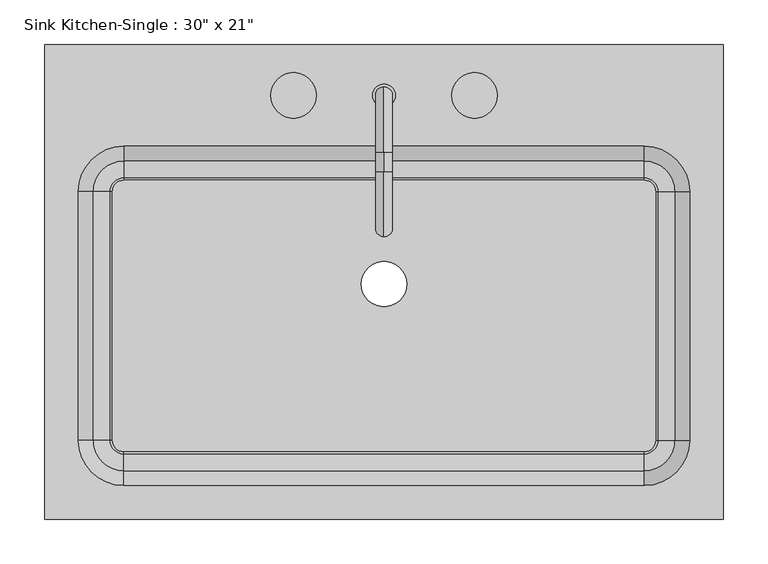
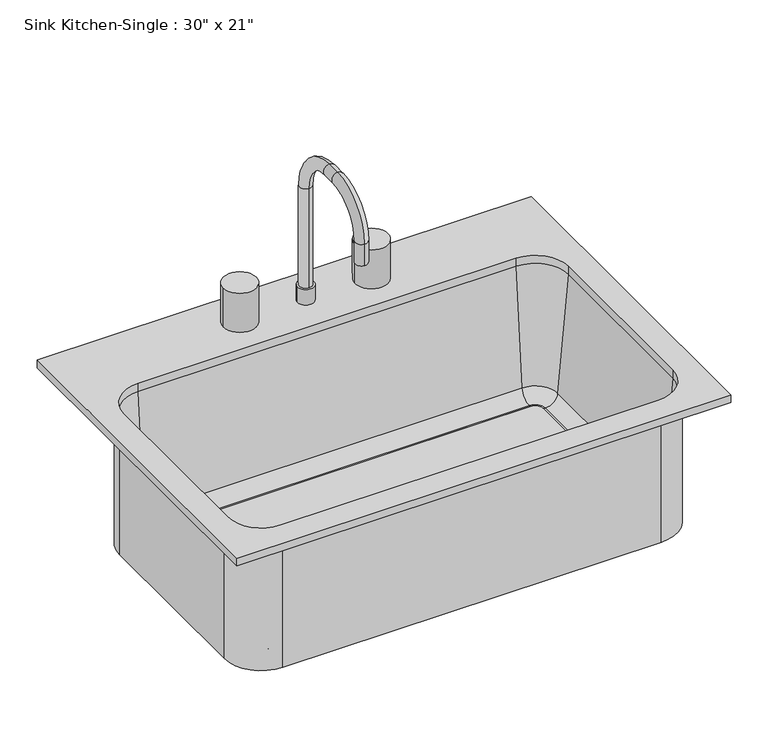
"""IFC4 building model written with IfcOpenShell, lengths in millimetres: flow terminal geometry."""

from ifc_helpers import new_model, si_unit, point, frame, frame_2d, origin, place, context, project, spatial, polyline, circle_curve, ellipse_curve, trimmed, segment, composite_curve, outline, extrude, source, transform, mapped, element, save
from ifc_brep_helpers import plane_surface, cylinder_surface, revolved_surface, advanced_brep


def flow_terminal_4d548711(model_context):
    return source(origin(), model_context, "Body", "SolidModel", [
        extrude(outline(composite_curve([segment(trimmed(circle_curve(frame_2d((307.7892406, 103.9454011)), 12.7), [point((307.7892406, 116.6454011))], [point((320.4892406, 103.9454011))], False, "CARTESIAN"), True, "CONTINUOUS"), segment(polyline([(320.4892406, 103.9454011), (320.4892406, -175.4545989)]), True, "CONTINUOUS"), segment(trimmed(circle_curve(frame_2d((307.7892406, -175.4545989)), 12.7), [point((320.4892406, -175.4545989))], [point((307.7892406, -188.1545989))], False, "CARTESIAN"), True, "CONTINUOUS"), segment(polyline([(307.7892406, -188.1545989), (-276.4107594, -188.1545989)]), True, "CONTINUOUS"), segment(trimmed(circle_curve(frame_2d((-276.4107594, -175.4545989)), 12.7), [point((-276.4107594, -188.1545989))], [point((-289.1107594, -175.4545989))], False, "CARTESIAN"), True, "CONTINUOUS"), segment(polyline([(-289.1107594, -175.4545989), (-289.1107594, 103.9454011)]), True, "CONTINUOUS"), segment(trimmed(circle_curve(frame_2d((-276.4107594, 103.9454011)), 12.7), [point((-289.1107594, 103.9454011))], [point((-276.4107594, 116.6454011))], False, "CARTESIAN"), True, "CONTINUOUS"), segment(polyline([(-276.4107594, 116.6454011), (307.7892406, 116.6454011)]), True, "CONTINUOUS")], self_intersect=False), holes=[composite_curve([segment(trimmed(circle_curve(frame_2d((15.6892406, 0.0)), 25.4), [point((-9.7107594, 0.0))], [point((41.0892406, 0.0))], True, "CARTESIAN"), True, "CONTINUOUS"), segment(trimmed(circle_curve(frame_2d((15.6892406, 0.0)), 25.4), [point((41.0892406, 0.0))], [point((-9.7107594, 0.0))], True, "CARTESIAN"), True, "CONTINUOUS")], self_intersect=False)]), frame((0.0, 0.0, 698.5), z_axis=(0.0, 0.0, 1.0), x_axis=(1.0, 0.0, 0.0)), (0.0, 0.0, 1.0), 9.525),
        extrude(outline(composite_curve([segment(trimmed(circle_curve(frame_2d((-85.9107594, 211.8954011)), 25.4), [point((-111.3107594, 211.8954011))], [point((-60.5107594, 211.8954011))], False, "CARTESIAN"), True, "CONTINUOUS"), segment(trimmed(circle_curve(frame_2d((-85.9107594, 211.8954011)), 25.4), [point((-60.5107594, 211.8954011))], [point((-111.3107594, 211.8954011))], False, "CARTESIAN"), True, "CONTINUOUS")], self_intersect=False)), frame((0.0, 0.0, 927.1), z_axis=(0.0, 0.0, 1.0), x_axis=(1.0, 0.0, 0.0)), (0.0, 0.0, 1.0), 63.5),
        extrude(outline(composite_curve([segment(trimmed(circle_curve(frame_2d((117.2892406, 211.8954011)), 25.4), [point((91.8892406, 211.8954011))], [point((142.6892406, 211.8954011))], False, "CARTESIAN"), True, "CONTINUOUS"), segment(trimmed(circle_curve(frame_2d((117.2892406, 211.8954011)), 25.4), [point((142.6892406, 211.8954011))], [point((91.8892406, 211.8954011))], False, "CARTESIAN"), True, "CONTINUOUS")], self_intersect=False)), frame((0.0, 0.0, 927.1), z_axis=(0.0, 0.0, 1.0), x_axis=(1.0, 0.0, 0.0)), (0.0, 0.0, 1.0), 63.5),
        advanced_brep(
        [(2.9892406, 211.8954011, 927.1), (28.3892406, 211.8954011, 927.1), (15.6892406, 221.4204011, 1114.425), (15.6892406, 202.3704011, 1114.425), (15.6892406, 202.3704011, 952.5), (15.6892406, 221.4204011, 952.5), (15.6892406, 148.3954011, 1187.45), (15.6892406, 148.3954011, 1168.4), (15.6892406, 126.1704011, 1187.45), (15.6892406, 126.1704011, 1168.4), (15.6892406, 53.1454011, 1114.425), (15.6892406, 72.1954011, 1114.425), (15.6892406, 53.1454011, 1079.5), (15.6892406, 72.1954011, 1079.5), (2.9892406, 211.8954011, 952.5), (28.3892406, 211.8954011, 952.5)],
        [
            (0, 1, circle_curve(frame((15.6892406, 211.8954011, 927.1), z_axis=(0.0, 0.0, -1.0), x_axis=(1.0, 0.0, 0.0)), 12.7)),
            (1, 0, circle_curve(frame((15.6892406, 211.8954011, 927.1), z_axis=(0.0, 0.0, -1.0), x_axis=(1.0, 0.0, 0.0)), 12.7)),
            (2, 3, circle_curve(frame((15.6892406, 211.8954011, 1114.425), z_axis=(0.0, 0.0, -1.0), x_axis=(0.0, -1.0, 0.0)), 9.525)),
            (3, 4),
            (4, 5, circle_curve(frame((15.6892406, 211.8954011, 952.5), z_axis=(0.0, 0.0, 1.0), x_axis=(0.0, -1.0, 0.0)), 9.525)),
            (5, 2),
            (3, 2, circle_curve(frame((15.6892406, 211.8954011, 1114.425), z_axis=(0.0, 0.0, -1.0), x_axis=(0.0, -1.0, 0.0)), 9.525)),
            (5, 4, circle_curve(frame((15.6892406, 211.8954011, 952.5), z_axis=(0.0, 0.0, 1.0), x_axis=(0.0, -1.0, 0.0)), 9.525)),
            (2, 6, circle_curve(frame((15.6892406, 148.3954011, 1114.425), z_axis=(1.0, 0.0, 0.0), x_axis=(0.0, 1.0, 0.0)), 73.025)),
            (6, 7, circle_curve(frame((15.6892406, 148.3954011, 1177.925), z_axis=(0.0, 1.0, 0.0), x_axis=(0.0, 0.0, -1.0)), 9.525)),
            (7, 3, circle_curve(frame((15.6892406, 148.3954011, 1114.425), z_axis=(-1.0, 0.0, 0.0), x_axis=(0.0, 1.0, 0.0)), 53.975)),
            (7, 6, circle_curve(frame((15.6892406, 148.3954011, 1177.925), z_axis=(0.0, 1.0, 0.0), x_axis=(0.0, 0.0, -1.0)), 9.525)),
            (6, 8),
            (8, 9, circle_curve(frame((15.6892406, 126.1704011, 1177.925), z_axis=(0.0, 1.0, 0.0), x_axis=(0.0, 0.0, -1.0)), 9.525)),
            (9, 7),
            (9, 8, circle_curve(frame((15.6892406, 126.1704011, 1177.925), z_axis=(0.0, 1.0, 0.0), x_axis=(0.0, 0.0, -1.0)), 9.525)),
            (8, 10, circle_curve(frame((15.6892406, 126.1704011, 1114.425), z_axis=(1.0, 0.0, 0.0), x_axis=(0.0, 0.0, 1.0)), 73.025)),
            (10, 11, circle_curve(frame((15.6892406, 62.6704011, 1114.425), z_axis=(0.0, 0.0, 1.0), x_axis=(0.0, 1.0, 0.0)), 9.525)),
            (11, 9, circle_curve(frame((15.6892406, 126.1704011, 1114.425), z_axis=(-1.0, 0.0, 0.0), x_axis=(0.0, 0.0, 1.0)), 53.975)),
            (11, 10, circle_curve(frame((15.6892406, 62.6704011, 1114.425), z_axis=(0.0, 0.0, 1.0), x_axis=(0.0, 1.0, 0.0)), 9.525)),
            (12, 13, circle_curve(frame((15.6892406, 62.6704011, 1079.5), z_axis=(0.0, 0.0, -1.0), x_axis=(0.0, 1.0, 0.0)), 9.525)),
            (13, 12, circle_curve(frame((15.6892406, 62.6704011, 1079.5), z_axis=(0.0, 0.0, -1.0), x_axis=(0.0, 1.0, 0.0)), 9.525)),
            (10, 12),
            (13, 11),
            (14, 15, circle_curve(frame((15.6892406, 211.8954011, 952.5), z_axis=(0.0, 0.0, 1.0), x_axis=(1.0, 0.0, 0.0)), 12.7)),
            (15, 14, circle_curve(frame((15.6892406, 211.8954011, 952.5), z_axis=(0.0, 0.0, 1.0), x_axis=(1.0, 0.0, 0.0)), 12.7)),
            (14, 0),
            (1, 15),
        ],
        [
            plane_surface(frame((15.6892406, 202.3704011, 927.1), z_axis=(0.0, 0.0, -1.0), x_axis=(1.0, 0.0, 0.0))),
            cylinder_surface(frame((15.6892406, 211.8954011, 927.1), z_axis=(0.0, 0.0, -1.0), x_axis=(0.0, -1.0, 0.0)), 9.525),
            revolved_surface(trimmed(ellipse_curve(frame((15.6892406, 211.8954011, 1114.425), z_axis=(0.0, 0.0, -1.0), x_axis=(0.0, -1.0, 0.0)), 9.525, 9.525), [point((15.6892406, 221.4204011, 1114.425))], [point((15.6892406, 202.3704011, 1114.425))], True, "CARTESIAN"), (15.6892406, 148.3954011, 1114.425), (1.0, 0.0, 0.0)),
            revolved_surface(trimmed(ellipse_curve(frame((15.6892406, 211.8954011, 1114.425), z_axis=(0.0, 0.0, -1.0), x_axis=(0.0, -1.0, 0.0)), 9.525, 9.525), [point((15.6892406, 202.3704011, 1114.425))], [point((15.6892406, 221.4204011, 1114.425))], True, "CARTESIAN"), (15.6892406, 148.3954011, 1114.425), (1.0, 0.0, 0.0)),
            cylinder_surface(frame((15.6892406, 148.3954011, 1177.925), z_axis=(0.0, 1.0, 0.0), x_axis=(0.0, 0.0, -1.0)), 9.525),
            revolved_surface(trimmed(ellipse_curve(frame((15.6892406, 126.1704011, 1177.925), z_axis=(0.0, 1.0, 0.0), x_axis=(0.0, 0.0, -1.0)), 9.525, 9.525), [point((15.6892406, 126.1704011, 1187.45))], [point((15.6892406, 126.1704011, 1168.4))], True, "CARTESIAN"), (15.6892406, 126.1704011, 1114.425), (1.0, 0.0, 0.0)),
            revolved_surface(trimmed(ellipse_curve(frame((15.6892406, 126.1704011, 1177.925), z_axis=(0.0, 1.0, 0.0), x_axis=(0.0, 0.0, -1.0)), 9.525, 9.525), [point((15.6892406, 126.1704011, 1168.4))], [point((15.6892406, 126.1704011, 1187.45))], True, "CARTESIAN"), (15.6892406, 126.1704011, 1114.425), (1.0, 0.0, 0.0)),
            plane_surface(frame((15.6892406, 53.1454011, 1079.5), z_axis=(0.0, 0.0, -1.0), x_axis=(-1.0, 0.0, 0.0))),
            cylinder_surface(frame((15.6892406, 62.6704011, 1114.425), z_axis=(0.0, 0.0, 1.0), x_axis=(0.0, 1.0, 0.0)), 9.525),
            plane_surface(frame((28.3892406, 211.8954011, 952.5), z_axis=(0.0, 0.0, 1.0), x_axis=(0.0, 1.0, 0.0))),
            cylinder_surface(frame((15.6892406, 211.8954011, 927.1), z_axis=(0.0, 0.0, 1.0), x_axis=(1.0, 0.0, 0.0)), 12.7),
        ],
        [
            (0, [[1, 2]]),
            (1, [[3, 4, 5, 6]]),
            (1, [[7, -6, 8, -4]]),
            (2, [[-3, 9, 10, 11]]),
            (3, [[-7, -11, 12, -9]]),
            (4, [[-10, 13, 14, 15]]),
            (4, [[-12, -15, 16, -13]]),
            (5, [[-14, 17, 18, 19]]),
            (6, [[-16, -19, 20, -17]]),
            (7, [[21, 22]]),
            (8, [[-18, 23, -22, 24]]),
            (8, [[-20, -24, -21, -23]]),
            (9, [[25, 26], [-5, -8]]),
            (10, [[-25, 27, -2, 28]]),
            (10, [[-26, -28, -1, -27]]),
        ],
    ),
        advanced_brep(
        [(396.6892406, 269.0454011, 927.1), (-365.3107594, 269.0454011, 927.1), (-365.3107594, -264.3545989, 927.1), (396.6892406, -264.3545989, 927.1), (307.7892406, 154.7454011, 927.1), (358.5892406, 103.9454011, 927.1), (358.5892406, -175.4545989, 927.1), (307.7892406, -226.2545989, 927.1), (-276.4107594, -226.2545989, 927.1), (-327.2107594, -175.4545989, 927.1), (-327.2107594, 103.9454011, 927.1), (-276.4107594, 154.7454011, 927.1), (396.6892406, 269.0454011, 914.4), (396.6892406, -264.3545989, 914.4), (-365.3107594, -264.3545989, 914.4), (-365.3107594, 269.0454011, 914.4), (364.9392406, 103.9454011, 914.4), (307.7892406, 161.0954011, 914.4), (-276.4107594, 161.0954011, 914.4), (-333.5607594, 103.9454011, 914.4), (-333.5607594, -175.4545989, 914.4), (-276.4107594, -232.6045989, 914.4), (307.7892406, -232.6045989, 914.4), (364.9392406, -175.4545989, 914.4), (307.7892406, 154.7454011, 914.4), (358.5892406, 103.9454011, 914.4), (358.5892406, -175.4545989, 914.4), (307.7892406, -226.2545989, 914.4), (-276.4107594, -226.2545989, 914.4), (-327.2107594, -175.4545989, 914.4), (-327.2107594, 103.9454011, 914.4), (-276.4107594, 154.7454011, 914.4), (364.9392406, 103.9454011, 698.5), (307.7892406, 161.0954011, 698.5), (320.4892406, 103.9454011, 698.5), (307.7892406, 116.6454011, 698.5), (320.4892406, 103.9454011, 708.025), (307.7892406, 116.6454011, 708.025), (323.0776588, 103.9454011, 708.025), (307.7892406, 119.2338193, 708.025), (342.0551678, 103.9454011, 725.4146831), (307.7892406, 138.2113283, 725.4146831), (364.9392406, -175.4545989, 698.5), (320.4892406, -175.4545989, 698.5), (320.4892406, -175.4545989, 708.025), (323.0776588, -175.4545989, 708.025), (342.0551678, -175.4545989, 725.4146831), (307.7892406, -232.6045989, 698.5), (307.7892406, -188.1545989, 698.5), (307.7892406, -188.1545989, 708.025), (307.7892406, -190.7430171, 708.025), (307.7892406, -209.7205261, 725.4146831), (-276.4107594, -232.6045989, 698.5), (-276.4107594, -188.1545989, 698.5), (-276.4107594, -188.1545989, 708.025), (-276.4107594, -190.7430171, 708.025), (-276.4107594, -209.7205261, 725.4146831), (-333.5607594, -175.4545989, 698.5), (-289.1107594, -175.4545989, 698.5), (-289.1107594, -175.4545989, 708.025), (-291.6991776, -175.4545989, 708.025), (-310.6766866, -175.4545989, 725.4146831), (-333.5607594, 103.9454011, 698.5), (-289.1107594, 103.9454011, 698.5), (-289.1107594, 103.9454011, 708.025), (-291.6991776, 103.9454011, 708.025), (-310.6766866, 103.9454011, 725.4146831), (-276.4107594, 161.0954011, 698.5), (-276.4107594, 116.6454011, 698.5), (-276.4107594, 116.6454011, 708.025), (-276.4107594, 119.2338193, 708.025), (-276.4107594, 138.2113283, 725.4146831)],
        [
            (0, 1),
            (1, 2),
            (2, 3),
            (3, 0),
            (4, 5, circle_curve(frame((307.7892406, 103.9454011, 927.1), z_axis=(0.0, 0.0, -1.0), x_axis=(1.0, 0.0, 0.0)), 50.8)),
            (5, 6),
            (6, 7, circle_curve(frame((307.7892406, -175.4545989, 927.1), z_axis=(0.0, 0.0, -1.0), x_axis=(1.0, 0.0, 0.0)), 50.8)),
            (7, 8),
            (8, 9, circle_curve(frame((-276.4107594, -175.4545989, 927.1), z_axis=(0.0, 0.0, -1.0), x_axis=(1.0, 0.0, 0.0)), 50.8)),
            (9, 10),
            (10, 11, circle_curve(frame((-276.4107594, 103.9454011, 927.1), z_axis=(0.0, 0.0, -1.0), x_axis=(1.0, 0.0, 0.0)), 50.8)),
            (11, 4),
            (12, 13),
            (13, 14),
            (14, 15),
            (15, 12),
            (16, 17, circle_curve(frame((307.7892406, 103.9454011, 914.4), z_axis=(0.0, 0.0, 1.0), x_axis=(0.0, 1.0, 0.0)), 57.15)),
            (17, 18),
            (18, 19, circle_curve(frame((-276.4107594, 103.9454011, 914.4), z_axis=(0.0, 0.0, 1.0), x_axis=(-1.0, 0.0, 0.0)), 57.15)),
            (19, 20),
            (20, 21, circle_curve(frame((-276.4107594, -175.4545989, 914.4), z_axis=(0.0, 0.0, 1.0), x_axis=(0.0, -1.0, 0.0)), 57.15)),
            (21, 22),
            (22, 23, circle_curve(frame((307.7892406, -175.4545989, 914.4), z_axis=(0.0, 0.0, 1.0), x_axis=(1.0, 0.0, 0.0)), 57.15)),
            (23, 16),
            (0, 12),
            (15, 1),
            (14, 2),
            (13, 3),
            (4, 24),
            (24, 25, circle_curve(frame((307.7892406, 103.9454011, 914.4), z_axis=(0.0, 0.0, -1.0), x_axis=(1.0, 0.0, 0.0)), 50.8)),
            (25, 5),
            (25, 26),
            (26, 6),
            (26, 27, circle_curve(frame((307.7892406, -175.4545989, 914.4), z_axis=(0.0, 0.0, -1.0), x_axis=(1.0, 0.0, 0.0)), 50.8)),
            (27, 7),
            (27, 28),
            (28, 8),
            (28, 29, circle_curve(frame((-276.4107594, -175.4545989, 914.4), z_axis=(0.0, 0.0, -1.0), x_axis=(1.0, 0.0, 0.0)), 50.8)),
            (29, 9),
            (29, 30),
            (30, 10),
            (30, 31, circle_curve(frame((-276.4107594, 103.9454011, 914.4), z_axis=(0.0, 0.0, -1.0), x_axis=(1.0, 0.0, 0.0)), 50.8)),
            (31, 11),
            (31, 24),
            (32, 33, circle_curve(frame((307.7892406, 103.9454011, 698.5), z_axis=(0.0, 0.0, 1.0), x_axis=(0.0, 1.0, 0.0)), 57.15)),
            (33, 17),
            (16, 32),
            (32, 34),
            (34, 35, circle_curve(frame((307.7892406, 103.9454011, 698.5), z_axis=(0.0, 0.0, 1.0), x_axis=(0.0, 1.0, 0.0)), 12.7)),
            (35, 33),
            (34, 36),
            (36, 37, circle_curve(frame((307.7892406, 103.9454011, 708.025), z_axis=(0.0, 0.0, 1.0), x_axis=(0.0, 1.0, 0.0)), 12.7)),
            (37, 35),
            (36, 38),
            (38, 39, circle_curve(frame((307.7892406, 103.9454011, 708.025), z_axis=(0.0, 0.0, 1.0), x_axis=(0.0, 1.0, 0.0)), 15.2884182)),
            (39, 37),
            (38, 40, circle_curve(frame((323.0776588, 103.9454011, 727.075), z_axis=(0.0, -1.0, 0.0), x_axis=(1.0, 0.0, 0.0)), 19.05)),
            (40, 41, circle_curve(frame((307.7892406, 103.9454011, 725.4146831), z_axis=(0.0, 0.0, 1.0), x_axis=(0.0, 1.0, 0.0)), 34.2659272)),
            (41, 39, circle_curve(frame((307.7892406, 119.2338193, 727.075), z_axis=(-1.0, 0.0, 0.0), x_axis=(0.0, 1.0, 0.0)), 19.05)),
            (40, 25),
            (24, 41),
            (23, 42),
            (42, 32),
            (42, 43),
            (43, 34),
            (43, 44),
            (44, 36),
            (44, 45),
            (45, 38),
            (45, 46, circle_curve(frame((323.0776588, -175.4545989, 727.075), z_axis=(0.0, -1.0, 0.0), x_axis=(1.0, 0.0, 0.0)), 19.05)),
            (46, 40),
            (46, 26),
            (22, 47),
            (47, 42, circle_curve(frame((307.7892406, -175.4545989, 698.5), z_axis=(0.0, 0.0, 1.0), x_axis=(1.0, 0.0, 0.0)), 57.15)),
            (47, 48),
            (48, 43, circle_curve(frame((307.7892406, -175.4545989, 698.5), z_axis=(0.0, 0.0, 1.0), x_axis=(1.0, 0.0, 0.0)), 12.7)),
            (48, 49),
            (49, 44, circle_curve(frame((307.7892406, -175.4545989, 708.025), z_axis=(0.0, 0.0, 1.0), x_axis=(1.0, 0.0, 0.0)), 12.7)),
            (49, 50),
            (50, 45, circle_curve(frame((307.7892406, -175.4545989, 708.025), z_axis=(0.0, 0.0, 1.0), x_axis=(1.0, 0.0, 0.0)), 15.2884182)),
            (50, 51, circle_curve(frame((307.7892406, -190.7430171, 727.075), z_axis=(-1.0, 0.0, 0.0), x_axis=(0.0, -1.0, 0.0)), 19.05)),
            (51, 46, circle_curve(frame((307.7892406, -175.4545989, 725.4146831), z_axis=(0.0, 0.0, 1.0), x_axis=(1.0, 0.0, 0.0)), 34.2659272)),
            (51, 27),
            (21, 52),
            (52, 47),
            (52, 53),
            (53, 48),
            (53, 54),
            (54, 49),
            (54, 55),
            (55, 50),
            (55, 56, circle_curve(frame((-276.4107594, -190.7430171, 727.075), z_axis=(-1.0, 0.0, 0.0), x_axis=(0.0, -1.0, 0.0)), 19.05)),
            (56, 51),
            (56, 28),
            (20, 57),
            (57, 52, circle_curve(frame((-276.4107594, -175.4545989, 698.5), z_axis=(0.0, 0.0, 1.0), x_axis=(0.0, -1.0, 0.0)), 57.15)),
            (57, 58),
            (58, 53, circle_curve(frame((-276.4107594, -175.4545989, 698.5), z_axis=(0.0, 0.0, 1.0), x_axis=(0.0, -1.0, 0.0)), 12.7)),
            (58, 59),
            (59, 54, circle_curve(frame((-276.4107594, -175.4545989, 708.025), z_axis=(0.0, 0.0, 1.0), x_axis=(0.0, -1.0, 0.0)), 12.7)),
            (59, 60),
            (60, 55, circle_curve(frame((-276.4107594, -175.4545989, 708.025), z_axis=(0.0, 0.0, 1.0), x_axis=(0.0, -1.0, 0.0)), 15.2884182)),
            (60, 61, circle_curve(frame((-291.6991776, -175.4545989, 727.075), z_axis=(0.0, 1.0, 0.0), x_axis=(-1.0, 0.0, 0.0)), 19.05)),
            (61, 56, circle_curve(frame((-276.4107594, -175.4545989, 725.4146831), z_axis=(0.0, 0.0, 1.0), x_axis=(0.0, -1.0, 0.0)), 34.2659272)),
            (61, 29),
            (19, 62),
            (62, 57),
            (62, 63),
            (63, 58),
            (63, 64),
            (64, 59),
            (64, 65),
            (65, 60),
            (65, 66, circle_curve(frame((-291.6991776, 103.9454011, 727.075), z_axis=(0.0, 1.0, 0.0), x_axis=(-1.0, 0.0, 0.0)), 19.05)),
            (66, 61),
            (66, 30),
            (18, 67),
            (67, 62, circle_curve(frame((-276.4107594, 103.9454011, 698.5), z_axis=(0.0, 0.0, 1.0), x_axis=(-1.0, 0.0, 0.0)), 57.15)),
            (67, 68),
            (68, 63, circle_curve(frame((-276.4107594, 103.9454011, 698.5), z_axis=(0.0, 0.0, 1.0), x_axis=(-1.0, 0.0, 0.0)), 12.7)),
            (68, 69),
            (69, 64, circle_curve(frame((-276.4107594, 103.9454011, 708.025), z_axis=(0.0, 0.0, 1.0), x_axis=(-1.0, 0.0, 0.0)), 12.7)),
            (69, 70),
            (70, 65, circle_curve(frame((-276.4107594, 103.9454011, 708.025), z_axis=(0.0, 0.0, 1.0), x_axis=(-1.0, 0.0, 0.0)), 15.2884182)),
            (70, 71, circle_curve(frame((-276.4107594, 119.2338193, 727.075), z_axis=(1.0, 0.0, 0.0), x_axis=(0.0, 1.0, 0.0)), 19.05)),
            (71, 66, circle_curve(frame((-276.4107594, 103.9454011, 725.4146831), z_axis=(0.0, 0.0, 1.0), x_axis=(-1.0, 0.0, 0.0)), 34.2659272)),
            (71, 31),
            (33, 67),
            (35, 68),
            (37, 69),
            (39, 70),
            (41, 71),
        ],
        [
            plane_surface(frame((-365.3107594, 269.0454011, 927.1), z_axis=(0.0, 0.0, 1.0), x_axis=(-1.0, 0.0, 0.0))),
            plane_surface(frame((-365.3107594, 269.0454011, 914.4), z_axis=(0.0, 0.0, -1.0), x_axis=(1.0, 0.0, 0.0))),
            plane_surface(frame((396.6892406, 269.0454011, 927.1), z_axis=(0.0, 1.0, 0.0), x_axis=(0.0, 0.0, -1.0))),
            plane_surface(frame((-365.3107594, 269.0454011, 927.1), z_axis=(-1.0, 0.0, 0.0), x_axis=(0.0, 0.0, -1.0))),
            plane_surface(frame((-365.3107594, -264.3545989, 927.1), z_axis=(0.0, -1.0, 0.0), x_axis=(0.0, 0.0, -1.0))),
            plane_surface(frame((396.6892406, -264.3545989, 927.1), z_axis=(1.0, 0.0, 0.0), x_axis=(0.0, 0.0, -1.0))),
            revolved_surface(polyline([(358.58924060000004, 103.9454011, 914.4), (358.58924060000004, 103.9454011, 927.1)]), (307.7892406, 103.9454011, 0.0), (0.0, 0.0, -1.0)),
            plane_surface(frame((358.5892406, 103.9454011, 927.1), z_axis=(-1.0, 0.0, 0.0), x_axis=(0.0, 0.0, -1.0))),
            revolved_surface(polyline([(358.58924060000004, -175.4545989, 914.4), (358.58924060000004, -175.4545989, 927.1)]), (307.7892406, -175.4545989, 0.0), (0.0, 0.0, -1.0)),
            plane_surface(frame((307.7892406, -226.2545989, 927.1), z_axis=(0.0, 1.0, 0.0), x_axis=(0.0, 0.0, -1.0))),
            revolved_surface(polyline([(-225.6107594, -175.4545989, 914.4), (-225.6107594, -175.4545989, 927.1)]), (-276.4107594, -175.4545989, 0.0), (0.0, 0.0, -1.0)),
            plane_surface(frame((-327.2107594, -175.4545989, 927.1), z_axis=(1.0, 0.0, 0.0), x_axis=(0.0, 0.0, -1.0))),
            revolved_surface(polyline([(-225.6107594, 103.9454011, 914.4), (-225.6107594, 103.9454011, 927.1)]), (-276.4107594, 103.9454011, 0.0), (0.0, 0.0, -1.0)),
            plane_surface(frame((-276.4107594, 154.7454011, 927.1), z_axis=(0.0, -1.0, 0.0), x_axis=(0.0, 0.0, -1.0))),
            cylinder_surface(frame((307.7892406, 103.9454011, 0.0), z_axis=(0.0, 0.0, -1.0), x_axis=(0.0, 1.0, 0.0)), 57.15),
            plane_surface(frame((307.7892406, 103.9454011, 698.5), z_axis=(0.0, 0.0, -1.0), x_axis=(0.0, 1.0, 0.0))),
            revolved_surface(polyline([(307.7892406, 116.6454011, 698.5), (307.7892406, 116.6454011, 708.025)]), (307.7892406, 103.9454011, 0.0), (0.0, 0.0, -1.0)),
            plane_surface(frame((307.7892406, 103.9454011, 708.025), z_axis=(0.0, 0.0, 1.0), x_axis=(0.0, 1.0, 0.0))),
            revolved_surface(trimmed(ellipse_curve(frame((307.7892406, 119.2338193, 727.075), z_axis=(1.0, 0.0, 0.0), x_axis=(0.0, 1.0, 0.0)), 19.05, 19.05), [point((307.7892406, 119.2338193, 708.025))], [point((307.7892406, 138.2113283, 725.4146831))], True, "CARTESIAN"), (307.7892406, 103.9454011, 0.0), (0.0, 0.0, -1.0)),
            revolved_surface(polyline([(307.7892406, 138.2113283, 725.4146831), (307.7892406, 154.7454011, 914.4)]), (307.7892406, 103.9454011, 0.0), (0.0, 0.0, -1.0)),
            plane_surface(frame((364.9392406, 103.9454011, 914.4), z_axis=(1.0, 0.0, 0.0), x_axis=(0.0, -1.0, 0.0))),
            plane_surface(frame((364.9392406, 103.9454011, 698.5), z_axis=(0.0, 0.0, -1.0), x_axis=(0.0, -1.0, 0.0))),
            plane_surface(frame((320.4892406, 103.9454011, 698.5), z_axis=(-1.0, 0.0, 0.0), x_axis=(0.0, -1.0, 0.0))),
            plane_surface(frame((320.4892406, 103.9454011, 708.025), z_axis=(0.0, 0.0, 1.0), x_axis=(0.0, -1.0, 0.0))),
            revolved_surface(polyline([(342.1276588, -175.45459889999998, 727.075), (342.1276588, 103.9454011, 727.075)]), (323.0776588, 103.9454011, 727.075), (0.0, -1.0, 0.0)),
            plane_surface(frame((342.0551678, 103.9454011, 725.4146831), z_axis=(-0.9961946980917442, 0.0, 0.08715574274767306), x_axis=(0.0, -1.0, 0.0))),
            cylinder_surface(frame((307.7892406, -175.4545989, 0.0), z_axis=(0.0, 0.0, -1.0), x_axis=(1.0, 0.0, 0.0)), 57.15),
            plane_surface(frame((307.7892406, -175.4545989, 698.5), z_axis=(0.0, 0.0, -1.0), x_axis=(1.0, 0.0, 0.0))),
            revolved_surface(polyline([(320.4892406, -175.4545989, 698.5), (320.4892406, -175.4545989, 708.025)]), (307.7892406, -175.4545989, 0.0), (0.0, 0.0, -1.0)),
            plane_surface(frame((307.7892406, -175.4545989, 708.025), z_axis=(0.0, 0.0, 1.0), x_axis=(1.0, 0.0, 0.0))),
            revolved_surface(trimmed(ellipse_curve(frame((323.0776588, -175.4545989, 727.075), z_axis=(0.0, -1.0, 0.0), x_axis=(1.0, 0.0, 0.0)), 19.05, 19.05), [point((323.0776588, -175.4545989, 708.025))], [point((342.0551678, -175.4545989, 725.4146831))], True, "CARTESIAN"), (307.7892406, -175.4545989, 0.0), (0.0, 0.0, -1.0)),
            revolved_surface(polyline([(342.0551678, -175.4545989, 725.4146831), (358.5892406, -175.4545989, 914.4)]), (307.7892406, -175.4545989, 0.0), (0.0, 0.0, -1.0)),
            plane_surface(frame((307.7892406, -232.6045989, 914.4), z_axis=(0.0, -1.0, 0.0), x_axis=(-1.0, 0.0, 0.0))),
            plane_surface(frame((307.7892406, -232.6045989, 698.5), z_axis=(0.0, 0.0, -1.0), x_axis=(-1.0, 0.0, 0.0))),
            plane_surface(frame((307.7892406, -188.1545989, 698.5), z_axis=(0.0, 1.0, 0.0), x_axis=(-1.0, 0.0, 0.0))),
            plane_surface(frame((307.7892406, -188.1545989, 708.025), z_axis=(0.0, 0.0, 1.0), x_axis=(-1.0, 0.0, 0.0))),
            revolved_surface(polyline([(-276.4107594, -209.79301710000001, 727.075), (307.7892406, -209.79301710000001, 727.075)]), (307.7892406, -190.7430171, 727.075), (-1.0, 0.0, 0.0)),
            plane_surface(frame((307.7892406, -209.7205261, 725.4146831), z_axis=(0.0, 0.9961946980917442, 0.08715574274767306), x_axis=(-1.0, 0.0, 0.0))),
            cylinder_surface(frame((-276.4107594, -175.4545989, 0.0), z_axis=(0.0, 0.0, -1.0), x_axis=(0.0, -1.0, 0.0)), 57.15),
            plane_surface(frame((-276.4107594, -175.4545989, 698.5), z_axis=(0.0, 0.0, -1.0), x_axis=(0.0, -1.0, 0.0))),
            revolved_surface(polyline([(-276.4107594, -188.1545989, 698.5), (-276.4107594, -188.1545989, 708.025)]), (-276.4107594, -175.4545989, 0.0), (0.0, 0.0, -1.0)),
            plane_surface(frame((-276.4107594, -175.4545989, 708.025), z_axis=(0.0, 0.0, 1.0), x_axis=(0.0, -1.0, 0.0))),
            revolved_surface(trimmed(ellipse_curve(frame((-276.4107594, -190.7430171, 727.075), z_axis=(-1.0, 0.0, 0.0), x_axis=(0.0, -1.0, 0.0)), 19.05, 19.05), [point((-276.4107594, -190.7430171, 708.025))], [point((-276.4107594, -209.7205261, 725.4146831))], True, "CARTESIAN"), (-276.4107594, -175.4545989, 0.0), (0.0, 0.0, -1.0)),
            revolved_surface(polyline([(-276.4107594, -209.7205261, 725.4146831), (-276.4107594, -226.2545989, 914.4)]), (-276.4107594, -175.4545989, 0.0), (0.0, 0.0, -1.0)),
            plane_surface(frame((-333.5607594, -175.4545989, 914.4), z_axis=(-1.0, 0.0, 0.0), x_axis=(0.0, 1.0, 0.0))),
            plane_surface(frame((-333.5607594, -175.4545989, 698.5), z_axis=(0.0, 0.0, -1.0), x_axis=(0.0, 1.0, 0.0))),
            plane_surface(frame((-289.1107594, -175.4545989, 698.5), z_axis=(1.0, 0.0, 0.0), x_axis=(0.0, 1.0, 0.0))),
            plane_surface(frame((-289.1107594, -175.4545989, 708.025), z_axis=(0.0, 0.0, 1.0), x_axis=(0.0, 1.0, 0.0))),
            revolved_surface(polyline([(-310.7491776, 103.94540109999997, 727.075), (-310.7491776, -175.4545989, 727.075)]), (-291.6991776, -175.4545989, 727.075), (0.0, 1.0, 0.0)),
            plane_surface(frame((-310.6766866, -175.4545989, 725.4146831), z_axis=(0.9961946980917442, 0.0, 0.08715574274767306), x_axis=(0.0, 1.0, 0.0))),
            cylinder_surface(frame((-276.4107594, 103.9454011, 0.0), z_axis=(0.0, 0.0, -1.0), x_axis=(-1.0, 0.0, 0.0)), 57.15),
            plane_surface(frame((-276.4107594, 103.9454011, 698.5), z_axis=(0.0, 0.0, -1.0), x_axis=(-1.0, 0.0, 0.0))),
            revolved_surface(polyline([(-289.1107594, 103.9454011, 698.5), (-289.1107594, 103.9454011, 708.025)]), (-276.4107594, 103.9454011, 0.0), (0.0, 0.0, -1.0)),
            plane_surface(frame((-276.4107594, 103.9454011, 708.025), z_axis=(0.0, 0.0, 1.0), x_axis=(-1.0, 0.0, 0.0))),
            revolved_surface(trimmed(ellipse_curve(frame((-291.6991776, 103.9454011, 727.075), z_axis=(0.0, 1.0, 0.0), x_axis=(-1.0, 0.0, 0.0)), 19.05, 19.05), [point((-291.6991776, 103.9454011, 708.025))], [point((-310.6766866, 103.9454011, 725.4146831))], True, "CARTESIAN"), (-276.4107594, 103.9454011, 0.0), (0.0, 0.0, -1.0)),
            revolved_surface(polyline([(-310.6766866, 103.9454011, 725.4146831), (-327.2107594, 103.9454011, 914.4)]), (-276.4107594, 103.9454011, 0.0), (0.0, 0.0, -1.0)),
            plane_surface(frame((-276.4107594, 161.0954011, 914.4), z_axis=(0.0, 1.0, 0.0), x_axis=(1.0, 0.0, 0.0))),
            plane_surface(frame((-276.4107594, 161.0954011, 698.5), z_axis=(0.0, 0.0, -1.0), x_axis=(1.0, 0.0, 0.0))),
            plane_surface(frame((-276.4107594, 116.6454011, 698.5), z_axis=(0.0, -1.0, 0.0), x_axis=(1.0, 0.0, 0.0))),
            plane_surface(frame((-276.4107594, 116.6454011, 708.025), z_axis=(0.0, 0.0, 1.0), x_axis=(1.0, 0.0, 0.0))),
            revolved_surface(polyline([(307.7892406, 138.2838193, 727.075), (-276.4107594, 138.2838193, 727.075)]), (-276.4107594, 119.2338193, 727.075), (1.0, 0.0, 0.0)),
            plane_surface(frame((-276.4107594, 138.2113283, 725.4146831), z_axis=(0.0, -0.9961946980917442, 0.08715574274767306), x_axis=(1.0, 0.0, 0.0))),
        ],
        [
            (0, [[1, 2, 3, 4], [5, 6, 7, 8, 9, 10, 11, 12]]),
            (1, [[13, 14, 15, 16], [17, 18, 19, 20, 21, 22, 23, 24]]),
            (2, [[-1, 25, -16, 26]]),
            (3, [[-2, -26, -15, 27]]),
            (4, [[-3, -27, -14, 28]]),
            (5, [[-4, -28, -13, -25]]),
            (6, [[-5, 29, 30, 31]]),
            (7, [[-6, -31, 32, 33]]),
            (8, [[-7, -33, 34, 35]]),
            (9, [[-8, -35, 36, 37]]),
            (10, [[-9, -37, 38, 39]]),
            (11, [[-10, -39, 40, 41]]),
            (12, [[-11, -41, 42, 43]]),
            (13, [[-12, -43, 44, -29]]),
            (14, [[45, 46, -17, 47]]),
            (15, [[-45, 48, 49, 50]]),
            (16, [[-49, 51, 52, 53]]),
            (17, [[-52, 54, 55, 56]]),
            (18, [[-55, 57, 58, 59]]),
            (19, [[-58, 60, -30, 61]]),
            (20, [[-47, -24, 62, 63]]),
            (21, [[-48, -63, 64, 65]]),
            (22, [[-51, -65, 66, 67]]),
            (23, [[-54, -67, 68, 69]]),
            (24, [[-57, -69, 70, 71]]),
            (25, [[-60, -71, 72, -32]]),
            (26, [[-62, -23, 73, 74]]),
            (27, [[-64, -74, 75, 76]]),
            (28, [[-66, -76, 77, 78]]),
            (29, [[-68, -78, 79, 80]]),
            (30, [[-70, -80, 81, 82]]),
            (31, [[-72, -82, 83, -34]]),
            (32, [[-73, -22, 84, 85]]),
            (33, [[-75, -85, 86, 87]]),
            (34, [[-77, -87, 88, 89]]),
            (35, [[-79, -89, 90, 91]]),
            (36, [[-81, -91, 92, 93]]),
            (37, [[-83, -93, 94, -36]]),
            (38, [[-84, -21, 95, 96]]),
            (39, [[-86, -96, 97, 98]]),
            (40, [[-88, -98, 99, 100]]),
            (41, [[-90, -100, 101, 102]]),
            (42, [[-92, -102, 103, 104]]),
            (43, [[-94, -104, 105, -38]]),
            (44, [[-95, -20, 106, 107]]),
            (45, [[-97, -107, 108, 109]]),
            (46, [[-99, -109, 110, 111]]),
            (47, [[-101, -111, 112, 113]]),
            (48, [[-103, -113, 114, 115]]),
            (49, [[-105, -115, 116, -40]]),
            (50, [[-106, -19, 117, 118]]),
            (51, [[-108, -118, 119, 120]]),
            (52, [[-110, -120, 121, 122]]),
            (53, [[-112, -122, 123, 124]]),
            (54, [[-114, -124, 125, 126]]),
            (55, [[-116, -126, 127, -42]]),
            (56, [[-46, 128, -117, -18]]),
            (57, [[-50, 129, -119, -128]]),
            (58, [[-53, 130, -121, -129]]),
            (59, [[-56, 131, -123, -130]]),
            (60, [[-59, 132, -125, -131]]),
            (61, [[-61, -44, -127, -132]]),
        ],
    ),
    ])


if __name__ == "__main__":
    model = new_model("IFC4")
    model_context = context("Model", 3, world=origin())
    ifc_project = project(units=[si_unit("LENGTHUNIT", "METRE", prefix="MILLI")], contexts=[model_context])
    site = spatial("IfcSite", under=ifc_project)
    building = spatial("IfcBuilding", under=site)
    placement = place(None, origin())
    flow_terminal_shape = flow_terminal_4d548711(model_context)
    element("IfcFlowTerminal", 1, ObjectType="Sink Kitchen-Single : 30\" x 21\"", at=placement, inside=building, context=model_context, shape_type="MappedRepresentation", body=[
        mapped(flow_terminal_shape, transform((0.0, 0.0, 0.0), x_axis=(1.0, 0.0, 0.0), y_axis=(0.0, 1.0, 0.0), z_axis=(0.0, 0.0, 1.0))),
    ])
    save(model, "model.ifc")

# Revit data of these elements
# Type "Sink Kitchen-Single : 30\" x 21\""
#   Assembly Code = "D2010410"
#   Counter Height = 3' - 0"
#   Depth = 1' - 9"
#   Width = 2' - 6"
#   Faucet Material = Steel, Polished
#   Sink Material = Steel, Polished
#   Default Elevation = 0
# Element 1 (IfcFlowTerminal, "Sink Kitchen-Single : 30\" x 21\"")
#   Materials on its faces: "Steel, Polished"
# Materials
#   "Steel, Polished": class "Metal", colour RGB 57 57 57, transparency 0, Description = "Polished steel", Cost = 0
